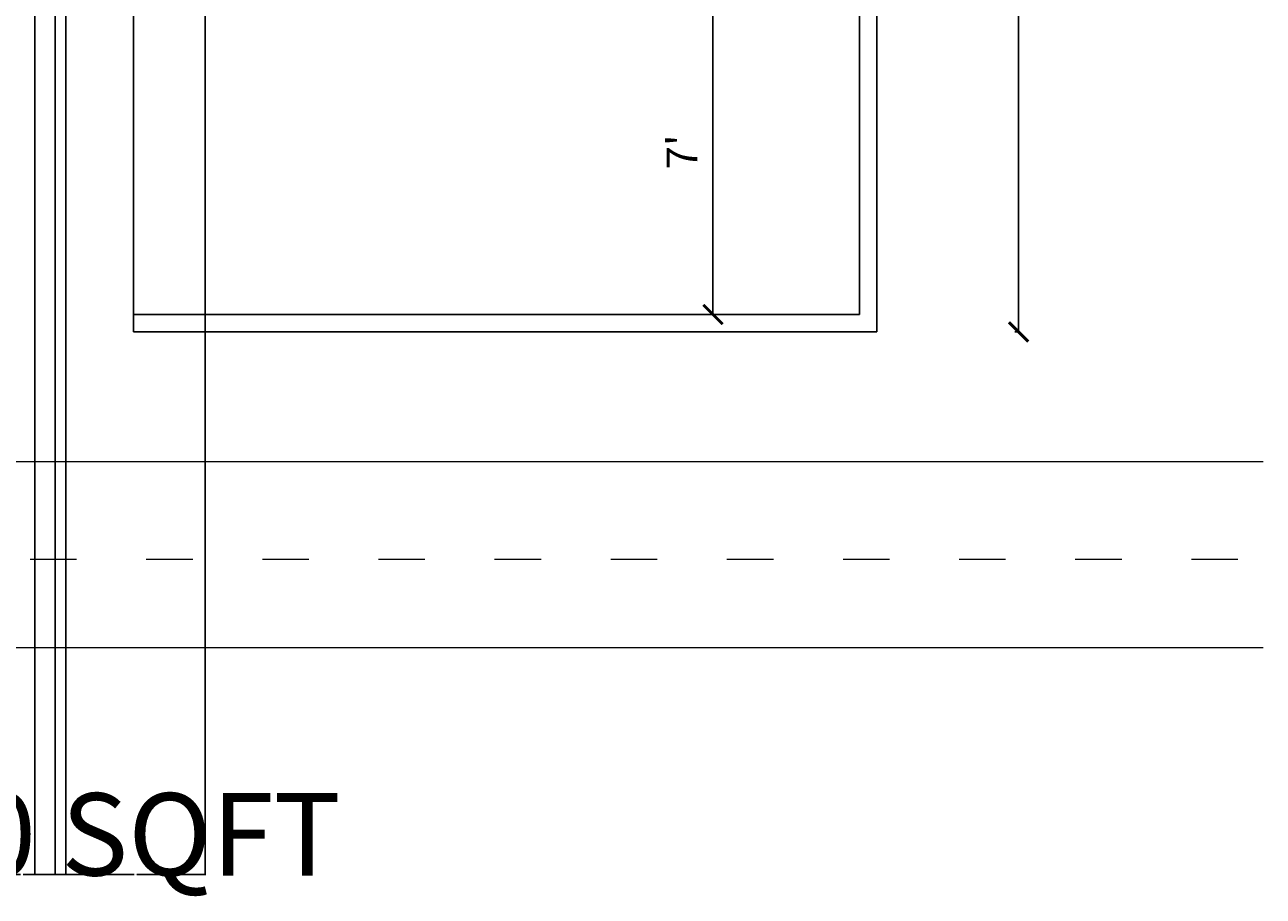
# Model space of a CAD drawing. Units: inches. Extents: x 502 to 1235, y -850 to 110.
# Tile 2 of 9: x 867 to 1187, y -850 to -625. Entities that reach past the tile are written whole.
import ezdxf

# ---------------------------------------------------------------- set-up
doc = ezdxf.new("R2010")
doc.units = ezdxf.units.IN
doc.header["$MEASUREMENT"] = 0
doc.linetypes.add('ACAD_ISO03W100', pattern=[30, 12, -18])
for name, color, linetype, lineweight in [('A-ANNO-DIMS', 2, 'Continuous', 18), ('A-AREA-IDEN', 8, 'Continuous', 18), ('C-PROP', 1, 'Continuous', 25), ('C-ROAD', 1, 'Continuous', 18), ('C-ROAD-CNTR', 1, 'ACAD_ISO03W100', 13)]:
    doc.layers.add(name, color=color, linetype=linetype, lineweight=lineweight)
doc.styles.get("Standard").update_dxf_attribs({"font": 'arial.ttf'})
doc.dimstyles.get("Standard").update_dxf_attribs({"dimtxt": 0.18, "dimasz": 0.18, "dimexe": 0.18, "dimexo": 0.0625, "dimgap": 0.09, "dimtad": 0, "dimtih": 1, "dimtoh": 1, "dimdec": 1, "dimzin": 0, "dimdsep": 46, "dimlunit": 4, "dimtxsty": 'Standard', "dimcen": 0.09, "dimadec": 0, "dimazin": 0, "dimtfac": 1, "dimtdec": 1, "dimtofl": 0, "dimtmove": 0, "dimatfit": 3, "dimfxl": 1, "dimtolj": 1, "dimtzin": 0, "dimarcsym": 0})

# ---------------------------------------------------------------- blocks, each defined once
blk = doc.blocks.new('_ArchTick')
at = {"color": 0, "linetype": 'ByBlock', "const_width": 0.15}
blk.add_lwpolyline([(-0.5, -0.5), (0.5, 0.5)], dxfattribs=at)
blk = doc.blocks.new('*D6')
at = {"layer": 'A-ANNO-DIMS', "color": 0, "lineweight": -2, "transparency": 16777216}
for p, q in [((1122.49, 15.65), (1123.67, 15.65)), ((1123.49, 15.65), (1123.49, -704.35)), ((1122.49, -704.35), (1123.67, -704.35))]:
    blk.add_line(p, q, dxfattribs=at)
at = {"layer": 'Defpoints', "color": 0, "transparency": 16777216}
for p in [(1086.89, 15.65), (1086.89, -704.35), (1123.49, -704.35)]:
    blk.add_point(p, dxfattribs=at)
at = {"layer": 'A-ANNO-DIMS', "color": 0, "lineweight": -2, "transparency": 16777216, "xscale": 5, "yscale": 5, "zscale": 5}
for p, rotation in [((1123.49, 15.65), 90), ((1123.49, -704.35), 270)]:
    blk.add_blockref('_ArchTick', p, dxfattribs=dict(at, rotation=rotation))
at = {"layer": 'A-ANNO-DIMS', "color": 0, "transparency": 16777216, "insert": (1115.41, -344.35), "char_height": 8, "attachment_point": 5, "rotation": 90}
blk.add_mtext("\\A1;60'", dxfattribs=at)
blk = doc.blocks.new('*D9')
at = {"layer": 'A-ANNO-DIMS', "color": 0, "lineweight": -2, "transparency": 16777216}
for p, q in [((1043.54, -615.85), (1044.72, -615.85)), ((1044.54, -615.85), (1044.54, -699.85)), ((1043.54, -699.85), (1044.72, -699.85))]:
    blk.add_line(p, q, dxfattribs=at)
at = {"layer": 'Defpoints', "color": 0, "transparency": 16777216}
for p in [(1010.39, -615.85), (1012.7, -699.85), (1044.54, -699.85)]:
    blk.add_point(p, dxfattribs=at)
at = {"layer": 'A-ANNO-DIMS', "color": 0, "lineweight": -2, "transparency": 16777216, "xscale": 5, "yscale": 5, "zscale": 5}
for p, rotation in [((1044.54, -615.85), 90), ((1044.54, -699.85), 270)]:
    blk.add_blockref('_ArchTick', p, dxfattribs=dict(at, rotation=rotation))
at = {"layer": 'A-ANNO-DIMS', "color": 0, "transparency": 16777216, "insert": (1036.54, -657.85), "char_height": 8, "attachment_point": 5, "rotation": 90}
blk.add_mtext("\\A1;7'", dxfattribs=at)
blk = doc.blocks.new('*D25')
at = {"layer": 'A-ANNO-DIMS', "color": 0, "lineweight": -2, "transparency": 16777216}
for p, q in [((798.89, -699.78), (798.89, 63.98)), ((894.89, -699.78), (894.89, 63.98)), ((799.07, 63.8), (846.56, 63.8)), ((894.71, 63.8), (847.22, 63.8))]:
    blk.add_line(p, q, dxfattribs=at)
at = {"layer": 'A-ANNO-DIMS', "color": 0, "transparency": 16777216}
for points in [[(799.07, 63.83), (799.07, 63.77), (798.89, 63.8)], [(894.71, 63.83), (894.71, 63.77), (894.89, 63.8)]]:
    blk.add_solid(points, dxfattribs=at)
at = {"layer": 'Defpoints', "color": 0, "transparency": 16777216}
for p in [(894.89, 63.8), (798.89, -699.85), (894.89, -699.85)]:
    blk.add_point(p, dxfattribs=at)
at = {"layer": 'A-ANNO-DIMS', "color": 0, "transparency": 16777216, "insert": (846.89, 63.8), "char_height": 0.18, "attachment_point": 5}
blk.add_mtext('\\A1;8\'-0"', dxfattribs=at)
blk = doc.blocks.new('*D41')
at = {"layer": 'A-ANNO-DIMS', "color": 0, "lineweight": -2, "transparency": 16777216}
for p, q in [((877.39, -422.41), (877.39, -844.7)), ((913.39, -422.41), (913.39, -844.7)), ((877.57, -844.52), (895.06, -844.52)), ((913.21, -844.52), (895.72, -844.52))]:
    blk.add_line(p, q, dxfattribs=at)
at = {"layer": 'A-ANNO-DIMS', "color": 0, "transparency": 16777216}
for points in [[(877.57, -844.49), (877.57, -844.55), (877.39, -844.52)], [(913.21, -844.49), (913.21, -844.55), (913.39, -844.52)]]:
    blk.add_solid(points, dxfattribs=at)
at = {"layer": 'Defpoints', "color": 0, "transparency": 16777216}
for p in [(877.39, -422.35), (913.39, -422.35), (913.39, -844.52)]:
    blk.add_point(p, dxfattribs=at)
at = {"layer": 'A-ANNO-DIMS', "color": 0, "transparency": 16777216, "insert": (895.39, -844.52), "char_height": 0.18, "attachment_point": 5}
blk.add_mtext('\\A1;3\'-0"', dxfattribs=at)
blk = doc.blocks.new('*D42')
at = {"layer": 'A-ANNO-DIMS', "color": 0, "lineweight": -2, "transparency": 16777216}
for p, q in [((869.39, -422.41), (869.39, -844.7)), ((877.39, -422.41), (877.39, -844.7)), ((869.57, -844.52), (873.06, -844.52)), ((877.21, -844.52), (873.72, -844.52))]:
    blk.add_line(p, q, dxfattribs=at)
at = {"layer": 'A-ANNO-DIMS', "color": 0, "transparency": 16777216}
for points in [[(869.57, -844.49), (869.57, -844.55), (869.39, -844.52)], [(877.21, -844.49), (877.21, -844.55), (877.39, -844.52)]]:
    blk.add_solid(points, dxfattribs=at)
at = {"layer": 'Defpoints', "color": 0, "transparency": 16777216}
for p in [(869.39, -422.35), (877.39, -422.35), (877.39, -844.52)]:
    blk.add_point(p, dxfattribs=at)
at = {"layer": 'A-ANNO-DIMS', "color": 0, "transparency": 16777216, "insert": (873.39, -844.52), "char_height": 0.18, "attachment_point": 5}
blk.add_mtext('\\A1;0\'-8"', dxfattribs=at)
blk = doc.blocks.new('*D47')
at = {"layer": 'A-ANNO-DIMS', "color": 0, "lineweight": -2, "transparency": 16777216}
for p, q in [((857.39, -551.41), (857.39, -844.7)), ((874.64, -551.41), (874.64, -844.7)), ((857.57, -844.52), (865.69, -844.52)), ((874.46, -844.52), (866.34, -844.52))]:
    blk.add_line(p, q, dxfattribs=at)
at = {"layer": 'A-ANNO-DIMS', "color": 0, "transparency": 16777216}
for points in [[(857.57, -844.49), (857.57, -844.55), (857.39, -844.52)], [(874.46, -844.49), (874.46, -844.55), (874.64, -844.52)]]:
    blk.add_solid(points, dxfattribs=at)
at = {"layer": 'Defpoints', "color": 0, "transparency": 16777216}
for p in [(857.39, -551.35), (874.64, -551.35), (874.64, -844.52)]:
    blk.add_point(p, dxfattribs=at)
at = {"layer": 'A-ANNO-DIMS', "color": 0, "transparency": 16777216, "insert": (866.01, -844.52), "char_height": 0.18, "attachment_point": 5}
blk.add_mtext('\\A1;1\'-5"', dxfattribs=at)

msp = doc.modelspace()

# ---------------------------------------------------------------- linework, layer by layer
at = {"layer": 'C-PROP'}
for p, q in [((1086.89, -704.35), (1086.89, 15.65)), ((1082.39, -699.85), (1082.39, 11.15)), ((894.89, -704.35), (894.89, -699.85)), ((894.89, -699.85), (1082.39, -699.85)), ((894.89, -704.35), (1086.89, -704.35))]:
    msp.add_line(p, q, dxfattribs=at)
at = {"layer": 'C-ROAD'}
for p, q in [((550.7, -737.83), (1186.68, -737.83)), ((550.7, -785.83), (1186.68, -785.83))]:
    msp.add_line(p, q, dxfattribs=at)
at = {"layer": 'C-ROAD-CNTR'}
msp.add_line((868.14, -763.02), (1185.25, -763.02), dxfattribs=at)

# ---------------------------------------------------------------- texts
at = {"layer": 'A-AREA-IDEN', "insert": (718.27, -823.48), "char_height": 21.2807, "attachment_point": 1}
msp.add_mtext_dynamic_manual_height_columns('AREA=1500 SQFT', width=263.9184, gutter_width=3.55, heights=[0], dxfattribs=at)

# ---------------------------------------------------------------- dimensions: what is measured, and where the dimension line sits
at = {"layer": 'A-ANNO-DIMS'}
for base, p1, p2, picture, middle in [((894.89, 63.8), (798.89, -699.85), (894.89, -699.85), '*D25', (846.89, 63.8)), ((877.39, -844.52), (869.39, -422.35), (877.39, -422.35), '*D42', (873.39, -844.52)), ((913.39, -844.52), (877.39, -422.35), (913.39, -422.35), '*D41', (895.39, -844.52)), ((874.6386, -844.5172), (857.3902, -551.3456), (874.6386, -551.3456), '*D47', (866.0144, -844.5172))]:
    dim = msp.add_linear_dim(base=base, p1=p1, p2=p2, dimstyle='Standard', override={"dimdec": 1, "dimlfac": 1, "dimrnd": 0, "dimzin": 1, "dimdsep": 46, "dimlunit": 4, "dimfrac": 2}, dxfattribs=at)
    dim.commit()
    dim.dimension.update_dxf_attribs({"geometry": picture, "text_midpoint": middle})
for base, p1, p2, picture, middle in [((1123.49, -704.35), (1086.89, 15.65), (1086.89, -704.35), '*D6', (1115.41, -344.35)), ((1044.54, -699.85), (1010.39, -615.85), (1012.7, -699.85), '*D9', (1036.54, -657.85))]:
    dim = msp.add_linear_dim(base=base, p1=p1, p2=p2, angle=90, dimstyle='Standard', override={"dimtxt": 8, "dimasz": 5, "dimgap": 4, "dimtad": 1, "dimtih": 0, "dimblk1": 'ArchTick', "dimblk2": 'ArchTick', "dimsah": 1, "dimclrd": 0, "dimclre": 0, "dimclrt": 0, "dimfxlon": 1}, dxfattribs=at)
    dim.commit()
    dim.dimension.update_dxf_attribs({"geometry": picture, "text_midpoint": middle})

doc.saveas('drawing.dxf')
